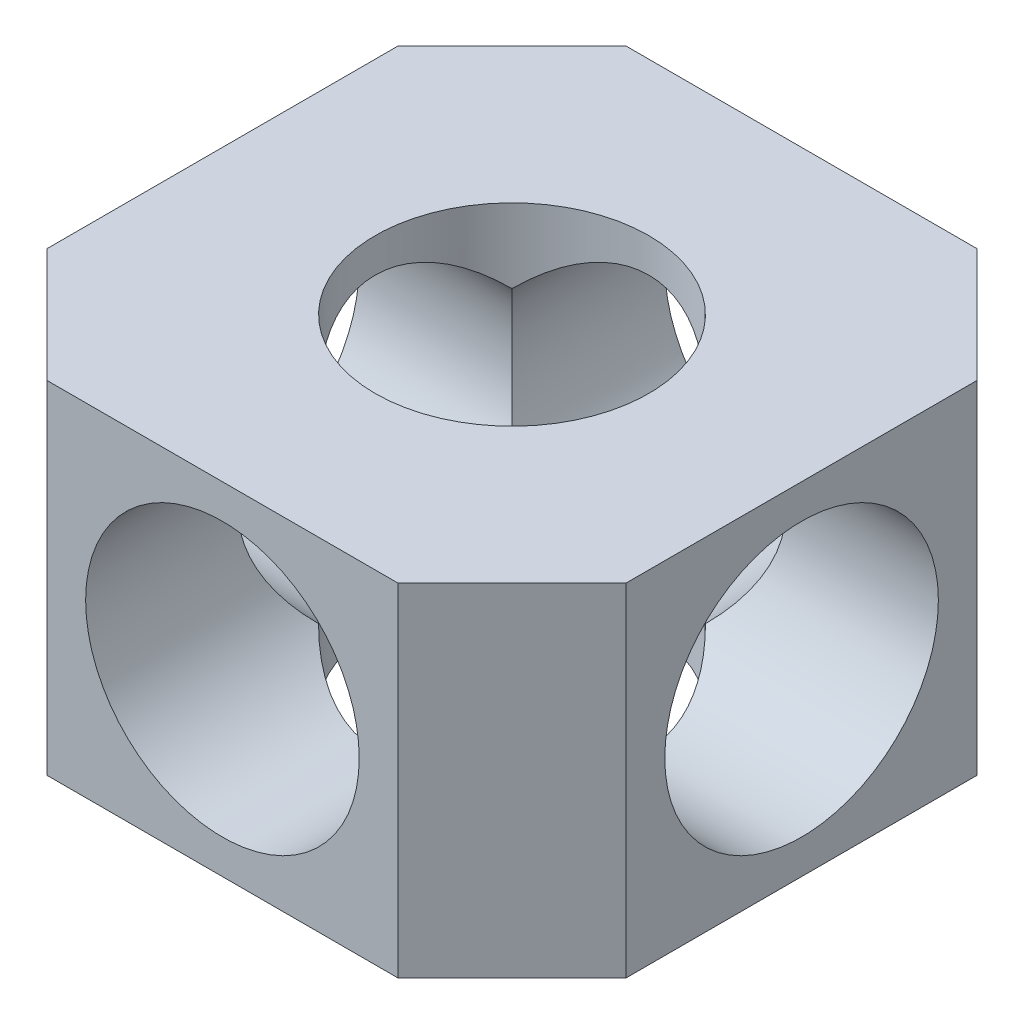
ISO-10303-21;
HEADER;
FILE_DESCRIPTION(('STEP AP214'),'2;1');
FILE_NAME('part.step','',(''),(''),'','','');
FILE_SCHEMA(('AUTOMOTIVE_DESIGN { 1 0 10303 214 1 1 1 1 }'));
ENDSEC;
DATA;
#1=APPLICATION_CONTEXT('core data for automotive mechanical design processes');
#2=APPLICATION_PROTOCOL_DEFINITION('international standard','automotive_design',2000,#1);
#3=PRODUCT_CONTEXT('',#1,'mechanical');
#4=PRODUCT('Part','Part','',(#3));
#5=PRODUCT_RELATED_PRODUCT_CATEGORY('part','',(#4));
#6=PRODUCT_DEFINITION_FORMATION('','',#4);
#7=PRODUCT_DEFINITION_CONTEXT('part definition',#1,'design');
#8=PRODUCT_DEFINITION('design','',#6,#7);
#9=PRODUCT_DEFINITION_SHAPE('','',#8);
#10=(LENGTH_UNIT() NAMED_UNIT(*) SI_UNIT(.MILLI.,.METRE.));
#11=(NAMED_UNIT(*) PLANE_ANGLE_UNIT() SI_UNIT($,.RADIAN.));
#12=(NAMED_UNIT(*) SI_UNIT($,.STERADIAN.) SOLID_ANGLE_UNIT());
#13=UNCERTAINTY_MEASURE_WITH_UNIT(LENGTH_MEASURE(1.E-05),#10,'distance_accuracy_value','');
#14=(GEOMETRIC_REPRESENTATION_CONTEXT(3) GLOBAL_UNCERTAINTY_ASSIGNED_CONTEXT((#13)) GLOBAL_UNIT_ASSIGNED_CONTEXT((#10,
#11,#12)) REPRESENTATION_CONTEXT('',''));
#15=CARTESIAN_POINT('',(0.,0.,0.));
#16=DIRECTION('',(0.,0.,1.));
#17=DIRECTION('',(1.,0.,0.));
#18=AXIS2_PLACEMENT_3D('',#15,#16,#17);
#19=CARTESIAN_POINT('',(0.,7.5,23.3));
#20=DIRECTION('',(0.,0.,-1.));
#21=DIRECTION('',(-1.,0.,0.));
#22=AXIS2_PLACEMENT_3D('',#19,#20,#21);
#23=CYLINDRICAL_SURFACE('',#22,6.);
#24=CARTESIAN_POINT('',(0.,7.5,-12.7));
#25=DIRECTION('',(0.,0.,-1.));
#26=DIRECTION('',(-1.,0.,0.));
#27=AXIS2_PLACEMENT_3D('',#24,#25,#26);
#28=CIRCLE('',#27,6.);
#29=CARTESIAN_POINT('',(-6.,7.5,-12.7));
#30=VERTEX_POINT('',#29);
#31=EDGE_CURVE('E179',#30,#30,#28,.T.);
#32=ORIENTED_EDGE('',*,*,#31,.T.);
#33=EDGE_LOOP('',(#32));
#34=FACE_BOUND('',#33,.T.);
#35=CARTESIAN_POINT('',(0.,7.5,0.));
#36=DIRECTION('',(0.707106781186547,0.,-0.707106781186548));
#37=DIRECTION('',(-0.707106781186548,0.,-0.707106781186547));
#38=AXIS2_PLACEMENT_3D('',#35,#36,#37);
#39=ELLIPSE('',#38,8.48528137423857,6.);
#40=CARTESIAN_POINT('',(-4.24264068711928,11.7426406871193,-4.24264068711928));
#41=VERTEX_POINT('',#40);
#42=CARTESIAN_POINT('',(-4.24264068711928,3.25735931288072,-4.24264068711928));
#43=VERTEX_POINT('',#42);
#44=EDGE_CURVE('E136',#41,#43,#39,.F.);
#45=ORIENTED_EDGE('',*,*,#44,.T.);
#46=CARTESIAN_POINT('',(0.,7.5,0.));
#47=DIRECTION('',(0.,0.707106781186547,-0.707106781186547));
#48=DIRECTION('',(0.,-0.707106781186547,-0.707106781186547));
#49=AXIS2_PLACEMENT_3D('',#46,#47,#48);
#50=ELLIPSE('',#49,8.48528137423857,6.);
#51=CARTESIAN_POINT('',(4.2426406871193,3.25735931288072,-4.24264068711928));
#52=VERTEX_POINT('',#51);
#53=EDGE_CURVE('E56',#43,#52,#50,.F.);
#54=ORIENTED_EDGE('',*,*,#53,.T.);
#55=CARTESIAN_POINT('',(0.,7.5,0.));
#56=DIRECTION('',(-0.707106781186548,0.,-0.707106781186547));
#57=DIRECTION('',(0.707106781186547,0.,-0.707106781186548));
#58=AXIS2_PLACEMENT_3D('',#55,#56,#57);
#59=ELLIPSE('',#58,8.48528137423857,6.);
#60=CARTESIAN_POINT('',(4.2426406871193,11.7426406871193,-4.24264068711928));
#61=VERTEX_POINT('',#60);
#62=EDGE_CURVE('E154',#52,#61,#59,.F.);
#63=ORIENTED_EDGE('',*,*,#62,.T.);
#64=CARTESIAN_POINT('',(0.,7.5,0.));
#65=DIRECTION('',(0.,-0.707106781186547,-0.707106781186547));
#66=DIRECTION('',(0.,0.707106781186547,-0.707106781186547));
#67=AXIS2_PLACEMENT_3D('',#64,#65,#66);
#68=ELLIPSE('',#67,8.48528137423857,6.);
#69=EDGE_CURVE('E162',#61,#41,#68,.F.);
#70=ORIENTED_EDGE('',*,*,#69,.T.);
#71=EDGE_LOOP('',(#45,#54,#63,#70));
#72=FACE_BOUND('',#71,.T.);
#73=ADVANCED_FACE('F43',(#34,#72),#23,.F.);
#74=CARTESIAN_POINT('',(12.7,15.,0.));
#75=DIRECTION('',(-1.,0.,0.));
#76=DIRECTION('',(0.,0.,1.));
#77=AXIS2_PLACEMENT_3D('',#74,#75,#76);
#78=PLANE('',#77);
#79=CARTESIAN_POINT('',(12.7,7.5,0.));
#80=DIRECTION('',(1.,0.,0.));
#81=DIRECTION('',(0.,0.,-1.));
#82=AXIS2_PLACEMENT_3D('',#79,#80,#81);
#83=CIRCLE('',#82,6.);
#84=CARTESIAN_POINT('',(12.7,7.5,-5.99999999999999));
#85=VERTEX_POINT('',#84);
#86=EDGE_CURVE('E172',#85,#85,#83,.T.);
#87=ORIENTED_EDGE('',*,*,#86,.F.);
#88=EDGE_LOOP('',(#87));
#89=FACE_BOUND('',#88,.T.);
#90=DIRECTION('',(0.,0.,-1.));
#91=VECTOR('',#90,1.);
#92=CARTESIAN_POINT('',(12.7,0.,0.));
#93=LINE('',#92,#91);
#94=CARTESIAN_POINT('',(12.7,0.,7.7));
#95=VERTEX_POINT('',#94);
#96=CARTESIAN_POINT('',(12.7,0.,-7.69999999999998));
#97=VERTEX_POINT('',#96);
#98=EDGE_CURVE('E196',#95,#97,#93,.T.);
#99=ORIENTED_EDGE('',*,*,#98,.T.);
#100=DIRECTION('',(0.,1.,0.));
#101=VECTOR('',#100,1.);
#102=CARTESIAN_POINT('',(12.7,15.,-7.69999999999998));
#103=LINE('',#102,#101);
#104=CARTESIAN_POINT('',(12.7,15.,-7.69999999999998));
#105=VERTEX_POINT('',#104);
#106=EDGE_CURVE('E225',#97,#105,#103,.T.);
#107=ORIENTED_EDGE('',*,*,#106,.T.);
#108=DIRECTION('',(0.,0.,-1.));
#109=VECTOR('',#108,1.);
#110=CARTESIAN_POINT('',(12.7,15.,12.7));
#111=LINE('',#110,#109);
#112=CARTESIAN_POINT('',(12.7,15.,7.7));
#113=VERTEX_POINT('',#112);
#114=EDGE_CURVE('E183',#113,#105,#111,.T.);
#115=ORIENTED_EDGE('',*,*,#114,.F.);
#116=DIRECTION('',(0.,-1.,0.));
#117=VECTOR('',#116,1.);
#118=CARTESIAN_POINT('',(12.7,15.,7.7));
#119=LINE('',#118,#117);
#120=EDGE_CURVE('E199',#113,#95,#119,.T.);
#121=ORIENTED_EDGE('',*,*,#120,.T.);
#122=EDGE_LOOP('',(#99,#107,#115,#121));
#123=FACE_BOUND('',#122,.T.);
#124=ADVANCED_FACE('F264',(#89,#123),#78,.F.);
#125=CARTESIAN_POINT('',(12.7,15.,-12.7));
#126=DIRECTION('',(0.,0.,1.));
#127=DIRECTION('',(1.,0.,0.));
#128=AXIS2_PLACEMENT_3D('',#125,#126,#127);
#129=PLANE('',#128);
#130=ORIENTED_EDGE('',*,*,#31,.F.);
#131=EDGE_LOOP('',(#130));
#132=FACE_BOUND('',#131,.T.);
#133=DIRECTION('',(-1.,0.,0.));
#134=VECTOR('',#133,1.);
#135=CARTESIAN_POINT('',(12.7,0.,-12.7));
#136=LINE('',#135,#134);
#137=CARTESIAN_POINT('',(7.7,0.,-12.7));
#138=VERTEX_POINT('',#137);
#139=CARTESIAN_POINT('',(-7.69999999999998,0.,-12.7));
#140=VERTEX_POINT('',#139);
#141=EDGE_CURVE('E197',#138,#140,#136,.T.);
#142=ORIENTED_EDGE('',*,*,#141,.T.);
#143=DIRECTION('',(0.,1.,0.));
#144=VECTOR('',#143,1.);
#145=CARTESIAN_POINT('',(-7.69999999999998,15.,-12.7));
#146=LINE('',#145,#144);
#147=CARTESIAN_POINT('',(-7.69999999999998,15.,-12.7));
#148=VERTEX_POINT('',#147);
#149=EDGE_CURVE('E233',#140,#148,#146,.T.);
#150=ORIENTED_EDGE('',*,*,#149,.T.);
#151=DIRECTION('',(-1.,0.,0.));
#152=VECTOR('',#151,1.);
#153=CARTESIAN_POINT('',(12.7,15.,-12.7));
#154=LINE('',#153,#152);
#155=CARTESIAN_POINT('',(7.7,15.,-12.7));
#156=VERTEX_POINT('',#155);
#157=EDGE_CURVE('E190',#156,#148,#154,.T.);
#158=ORIENTED_EDGE('',*,*,#157,.F.);
#159=DIRECTION('',(0.,-1.,0.));
#160=VECTOR('',#159,1.);
#161=CARTESIAN_POINT('',(7.7,15.,-12.7));
#162=LINE('',#161,#160);
#163=EDGE_CURVE('E216',#156,#138,#162,.T.);
#164=ORIENTED_EDGE('',*,*,#163,.T.);
#165=EDGE_LOOP('',(#142,#150,#158,#164));
#166=FACE_BOUND('',#165,.T.);
#167=ADVANCED_FACE('F266',(#132,#166),#129,.F.);
#168=CARTESIAN_POINT('',(-12.7,15.,-12.7));
#169=DIRECTION('',(1.,0.,0.));
#170=DIRECTION('',(0.,0.,-1.));
#171=AXIS2_PLACEMENT_3D('',#168,#169,#170);
#172=PLANE('',#171);
#173=CARTESIAN_POINT('',(-12.7,7.5,0.));
#174=DIRECTION('',(1.,0.,0.));
#175=DIRECTION('',(0.,0.,-1.));
#176=AXIS2_PLACEMENT_3D('',#173,#174,#175);
#177=CIRCLE('',#176,6.);
#178=CARTESIAN_POINT('',(-12.7,7.5,-5.99999999999999));
#179=VERTEX_POINT('',#178);
#180=EDGE_CURVE('E180',#179,#179,#177,.T.);
#181=ORIENTED_EDGE('',*,*,#180,.T.);
#182=EDGE_LOOP('',(#181));
#183=FACE_BOUND('',#182,.T.);
#184=DIRECTION('',(0.,0.,1.));
#185=VECTOR('',#184,1.);
#186=CARTESIAN_POINT('',(-12.7,0.,-12.7));
#187=LINE('',#186,#185);
#188=CARTESIAN_POINT('',(-12.7,0.,-7.69999999999999));
#189=VERTEX_POINT('',#188);
#190=CARTESIAN_POINT('',(-12.7,0.,7.69999999999999));
#191=VERTEX_POINT('',#190);
#192=EDGE_CURVE('E201',#189,#191,#187,.T.);
#193=ORIENTED_EDGE('',*,*,#192,.T.);
#194=DIRECTION('',(0.,1.,0.));
#195=VECTOR('',#194,1.);
#196=CARTESIAN_POINT('',(-12.7,15.,7.69999999999999));
#197=LINE('',#196,#195);
#198=CARTESIAN_POINT('',(-12.7,15.,7.69999999999999));
#199=VERTEX_POINT('',#198);
#200=EDGE_CURVE('E239',#191,#199,#197,.T.);
#201=ORIENTED_EDGE('',*,*,#200,.T.);
#202=DIRECTION('',(0.,0.,1.));
#203=VECTOR('',#202,1.);
#204=CARTESIAN_POINT('',(-12.7,15.,-12.7));
#205=LINE('',#204,#203);
#206=CARTESIAN_POINT('',(-12.7,15.,-7.69999999999999));
#207=VERTEX_POINT('',#206);
#208=EDGE_CURVE('E192',#207,#199,#205,.T.);
#209=ORIENTED_EDGE('',*,*,#208,.F.);
#210=DIRECTION('',(0.,-1.,0.));
#211=VECTOR('',#210,1.);
#212=CARTESIAN_POINT('',(-12.7,15.,-7.69999999999999));
#213=LINE('',#212,#211);
#214=EDGE_CURVE('E228',#207,#189,#213,.T.);
#215=ORIENTED_EDGE('',*,*,#214,.T.);
#216=EDGE_LOOP('',(#193,#201,#209,#215));
#217=FACE_BOUND('',#216,.T.);
#218=ADVANCED_FACE('F273',(#183,#217),#172,.F.);
#219=CARTESIAN_POINT('',(-12.7,15.,12.7));
#220=DIRECTION('',(0.,0.,-1.));
#221=DIRECTION('',(-1.,0.,0.));
#222=AXIS2_PLACEMENT_3D('',#219,#220,#221);
#223=PLANE('',#222);
#224=CARTESIAN_POINT('',(0.,7.5,12.7));
#225=DIRECTION('',(0.,0.,-1.));
#226=DIRECTION('',(-1.,0.,0.));
#227=AXIS2_PLACEMENT_3D('',#224,#225,#226);
#228=CIRCLE('',#227,6.);
#229=CARTESIAN_POINT('',(-5.99999999999999,7.5,12.7));
#230=VERTEX_POINT('',#229);
#231=EDGE_CURVE('E182',#230,#230,#228,.T.);
#232=ORIENTED_EDGE('',*,*,#231,.T.);
#233=EDGE_LOOP('',(#232));
#234=FACE_BOUND('',#233,.T.);
#235=DIRECTION('',(1.,0.,0.));
#236=VECTOR('',#235,1.);
#237=CARTESIAN_POINT('',(-12.7,15.,12.7));
#238=LINE('',#237,#236);
#239=CARTESIAN_POINT('',(-7.69999999999999,15.,12.7));
#240=VERTEX_POINT('',#239);
#241=CARTESIAN_POINT('',(7.69999999999998,15.,12.7));
#242=VERTEX_POINT('',#241);
#243=EDGE_CURVE('E191',#240,#242,#238,.T.);
#244=ORIENTED_EDGE('',*,*,#243,.F.);
#245=DIRECTION('',(0.,-1.,0.));
#246=VECTOR('',#245,1.);
#247=CARTESIAN_POINT('',(-7.69999999999999,15.,12.7));
#248=LINE('',#247,#246);
#249=CARTESIAN_POINT('',(-7.69999999999999,0.,12.7));
#250=VERTEX_POINT('',#249);
#251=EDGE_CURVE('E232',#240,#250,#248,.T.);
#252=ORIENTED_EDGE('',*,*,#251,.T.);
#253=DIRECTION('',(1.,0.,0.));
#254=VECTOR('',#253,1.);
#255=CARTESIAN_POINT('',(-12.7,0.,12.7));
#256=LINE('',#255,#254);
#257=CARTESIAN_POINT('',(7.69999999999998,0.,12.7));
#258=VERTEX_POINT('',#257);
#259=EDGE_CURVE('E189',#250,#258,#256,.T.);
#260=ORIENTED_EDGE('',*,*,#259,.T.);
#261=DIRECTION('',(0.,1.,0.));
#262=VECTOR('',#261,1.);
#263=CARTESIAN_POINT('',(7.69999999999998,15.,12.7));
#264=LINE('',#263,#262);
#265=EDGE_CURVE('E215',#258,#242,#264,.T.);
#266=ORIENTED_EDGE('',*,*,#265,.T.);
#267=EDGE_LOOP('',(#244,#252,#260,#266));
#268=FACE_BOUND('',#267,.T.);
#269=ADVANCED_FACE('F244',(#234,#268),#223,.F.);
#270=CARTESIAN_POINT('',(0.,15.,0.));
#271=DIRECTION('',(0.,1.,0.));
#272=DIRECTION('',(0.,0.,1.));
#273=AXIS2_PLACEMENT_3D('',#270,#271,#272);
#274=PLANE('',#273);
#275=CARTESIAN_POINT('',(0.,15.,0.));
#276=DIRECTION('',(0.,1.,0.));
#277=DIRECTION('',(0.,0.,1.));
#278=AXIS2_PLACEMENT_3D('',#275,#276,#277);
#279=CIRCLE('',#278,6.);
#280=CARTESIAN_POINT('',(0.,15.,6.));
#281=VERTEX_POINT('',#280);
#282=EDGE_CURVE('E150',#281,#281,#279,.T.);
#283=ORIENTED_EDGE('',*,*,#282,.F.);
#284=EDGE_LOOP('',(#283));
#285=FACE_BOUND('',#284,.T.);
#286=ORIENTED_EDGE('',*,*,#208,.T.);
#287=DIRECTION('',(-0.707106781186546,0.,-0.707106781186549));
#288=VECTOR('',#287,1.);
#289=CARTESIAN_POINT('',(-10.2,15.,10.2));
#290=LINE('',#289,#288);
#291=EDGE_CURVE('E152',#199,#240,#290,.F.);
#292=ORIENTED_EDGE('',*,*,#291,.T.);
#293=ORIENTED_EDGE('',*,*,#243,.T.);
#294=DIRECTION('',(-0.707106781186549,0.,0.707106781186547));
#295=VECTOR('',#294,1.);
#296=CARTESIAN_POINT('',(10.2,15.,10.2));
#297=LINE('',#296,#295);
#298=EDGE_CURVE('E213',#242,#113,#297,.F.);
#299=ORIENTED_EDGE('',*,*,#298,.T.);
#300=ORIENTED_EDGE('',*,*,#114,.T.);
#301=DIRECTION('',(0.707106781186546,0.,0.707106781186549));
#302=VECTOR('',#301,1.);
#303=CARTESIAN_POINT('',(10.2,15.,-10.2));
#304=LINE('',#303,#302);
#305=EDGE_CURVE('E224',#105,#156,#304,.F.);
#306=ORIENTED_EDGE('',*,*,#305,.T.);
#307=ORIENTED_EDGE('',*,*,#157,.T.);
#308=DIRECTION('',(0.707106781186549,0.,-0.707106781186546));
#309=VECTOR('',#308,1.);
#310=CARTESIAN_POINT('',(-10.2,15.,-10.2));
#311=LINE('',#310,#309);
#312=EDGE_CURVE('E231',#148,#207,#311,.F.);
#313=ORIENTED_EDGE('',*,*,#312,.T.);
#314=EDGE_LOOP('',(#286,#292,#293,#299,#300,#306,#307,#313));
#315=FACE_BOUND('',#314,.T.);
#316=ADVANCED_FACE('F290',(#285,#315),#274,.T.);
#317=CARTESIAN_POINT('',(0.,0.,0.));
#318=DIRECTION('',(0.,1.,0.));
#319=DIRECTION('',(0.,0.,1.));
#320=AXIS2_PLACEMENT_3D('',#317,#318,#319);
#321=PLANE('',#320);
#322=CARTESIAN_POINT('',(0.,0.,0.));
#323=DIRECTION('',(0.,1.,0.));
#324=DIRECTION('',(0.,0.,1.));
#325=AXIS2_PLACEMENT_3D('',#322,#323,#324);
#326=CIRCLE('',#325,6.);
#327=CARTESIAN_POINT('',(0.,0.,6.));
#328=VERTEX_POINT('',#327);
#329=EDGE_CURVE('E168',#328,#328,#326,.T.);
#330=ORIENTED_EDGE('',*,*,#329,.T.);
#331=EDGE_LOOP('',(#330));
#332=FACE_BOUND('',#331,.T.);
#333=ORIENTED_EDGE('',*,*,#259,.F.);
#334=DIRECTION('',(0.707106781186546,0.,0.707106781186549));
#335=VECTOR('',#334,1.);
#336=CARTESIAN_POINT('',(-7.69999999999999,0.,12.7));
#337=LINE('',#336,#335);
#338=EDGE_CURVE('E238',#250,#191,#337,.F.);
#339=ORIENTED_EDGE('',*,*,#338,.T.);
#340=ORIENTED_EDGE('',*,*,#192,.F.);
#341=DIRECTION('',(-0.707106781186549,0.,0.707106781186546));
#342=VECTOR('',#341,1.);
#343=CARTESIAN_POINT('',(-12.7,0.,-7.69999999999999));
#344=LINE('',#343,#342);
#345=EDGE_CURVE('E230',#189,#140,#344,.F.);
#346=ORIENTED_EDGE('',*,*,#345,.T.);
#347=ORIENTED_EDGE('',*,*,#141,.F.);
#348=DIRECTION('',(-0.707106781186546,0.,-0.707106781186549));
#349=VECTOR('',#348,1.);
#350=CARTESIAN_POINT('',(7.69999999999999,0.,-12.7));
#351=LINE('',#350,#349);
#352=EDGE_CURVE('E217',#138,#97,#351,.F.);
#353=ORIENTED_EDGE('',*,*,#352,.T.);
#354=ORIENTED_EDGE('',*,*,#98,.F.);
#355=DIRECTION('',(0.707106781186549,0.,-0.707106781186547));
#356=VECTOR('',#355,1.);
#357=CARTESIAN_POINT('',(12.7,0.,7.7));
#358=LINE('',#357,#356);
#359=EDGE_CURVE('E209',#95,#258,#358,.F.);
#360=ORIENTED_EDGE('',*,*,#359,.T.);
#361=EDGE_LOOP('',(#333,#339,#340,#346,#347,#353,#354,#360));
#362=FACE_BOUND('',#361,.T.);
#363=ADVANCED_FACE('F310',(#332,#362),#321,.F.);
#364=CARTESIAN_POINT('',(12.7,15.,7.7));
#365=DIRECTION('',(-0.707106781186547,0.,-0.707106781186549));
#366=DIRECTION('',(0.,-1.,0.));
#367=AXIS2_PLACEMENT_3D('',#364,#365,#366);
#368=PLANE('',#367);
#369=ORIENTED_EDGE('',*,*,#298,.F.);
#370=ORIENTED_EDGE('',*,*,#265,.F.);
#371=ORIENTED_EDGE('',*,*,#359,.F.);
#372=ORIENTED_EDGE('',*,*,#120,.F.);
#373=EDGE_LOOP('',(#369,#370,#371,#372));
#374=FACE_BOUND('',#373,.T.);
#375=ADVANCED_FACE('F299',(#374),#368,.F.);
#376=CARTESIAN_POINT('',(7.69999999999999,15.,-12.7));
#377=DIRECTION('',(-0.707106781186549,0.,0.707106781186546));
#378=DIRECTION('',(0.,-1.,0.));
#379=AXIS2_PLACEMENT_3D('',#376,#377,#378);
#380=PLANE('',#379);
#381=ORIENTED_EDGE('',*,*,#305,.F.);
#382=ORIENTED_EDGE('',*,*,#106,.F.);
#383=ORIENTED_EDGE('',*,*,#352,.F.);
#384=ORIENTED_EDGE('',*,*,#163,.F.);
#385=EDGE_LOOP('',(#381,#382,#383,#384));
#386=FACE_BOUND('',#385,.T.);
#387=ADVANCED_FACE('F306',(#386),#380,.F.);
#388=CARTESIAN_POINT('',(-12.7,15.,-7.69999999999999));
#389=DIRECTION('',(0.707106781186546,0.,0.707106781186549));
#390=DIRECTION('',(0.,-1.,0.));
#391=AXIS2_PLACEMENT_3D('',#388,#389,#390);
#392=PLANE('',#391);
#393=ORIENTED_EDGE('',*,*,#312,.F.);
#394=ORIENTED_EDGE('',*,*,#149,.F.);
#395=ORIENTED_EDGE('',*,*,#345,.F.);
#396=ORIENTED_EDGE('',*,*,#214,.F.);
#397=EDGE_LOOP('',(#393,#394,#395,#396));
#398=FACE_BOUND('',#397,.T.);
#399=ADVANCED_FACE('F260',(#398),#392,.F.);
#400=CARTESIAN_POINT('',(-7.69999999999999,15.,12.7));
#401=DIRECTION('',(0.707106781186549,0.,-0.707106781186546));
#402=DIRECTION('',(0.,-1.,0.));
#403=AXIS2_PLACEMENT_3D('',#400,#401,#402);
#404=PLANE('',#403);
#405=ORIENTED_EDGE('',*,*,#291,.F.);
#406=ORIENTED_EDGE('',*,*,#200,.F.);
#407=ORIENTED_EDGE('',*,*,#338,.F.);
#408=ORIENTED_EDGE('',*,*,#251,.F.);
#409=EDGE_LOOP('',(#405,#406,#407,#408));
#410=FACE_BOUND('',#409,.T.);
#411=ADVANCED_FACE('F46',(#410),#404,.F.);
#412=CARTESIAN_POINT('',(0.,7.5,0.));
#413=DIRECTION('',(-0.707106781186548,0.,-0.707106781186547));
#414=DIRECTION('',(0.707106781186547,0.,-0.707106781186548));
#415=AXIS2_PLACEMENT_3D('',#412,#413,#414);
#416=ELLIPSE('',#415,8.48528137423857,6.);
#417=CARTESIAN_POINT('',(-4.24264068711928,3.25735931288072,4.2426406871193));
#418=VERTEX_POINT('',#417);
#419=CARTESIAN_POINT('',(-4.24264068711928,11.7426406871193,4.2426406871193));
#420=VERTEX_POINT('',#419);
#421=EDGE_CURVE('E144',#418,#420,#416,.T.);
#422=ORIENTED_EDGE('',*,*,#421,.T.);
#423=CARTESIAN_POINT('',(0.,7.5,0.));
#424=DIRECTION('',(0.,0.707106781186547,-0.707106781186547));
#425=DIRECTION('',(0.,-0.707106781186547,-0.707106781186547));
#426=AXIS2_PLACEMENT_3D('',#423,#424,#425);
#427=ELLIPSE('',#426,8.48528137423857,6.);
#428=CARTESIAN_POINT('',(4.24264068711929,11.7426406871193,4.24264068711929));
#429=VERTEX_POINT('',#428);
#430=EDGE_CURVE('E66',#420,#429,#427,.T.);
#431=ORIENTED_EDGE('',*,*,#430,.T.);
#432=CARTESIAN_POINT('',(0.,7.5,0.));
#433=DIRECTION('',(0.707106781186547,0.,-0.707106781186548));
#434=DIRECTION('',(-0.707106781186548,0.,-0.707106781186547));
#435=AXIS2_PLACEMENT_3D('',#432,#433,#434);
#436=ELLIPSE('',#435,8.48528137423857,6.);
#437=CARTESIAN_POINT('',(4.24264068711929,3.25735931288071,4.24264068711929));
#438=VERTEX_POINT('',#437);
#439=EDGE_CURVE('E147',#429,#438,#436,.T.);
#440=ORIENTED_EDGE('',*,*,#439,.T.);
#441=CARTESIAN_POINT('',(0.,7.5,0.));
#442=DIRECTION('',(0.,-0.707106781186547,-0.707106781186547));
#443=DIRECTION('',(0.,0.707106781186547,-0.707106781186547));
#444=AXIS2_PLACEMENT_3D('',#441,#442,#443);
#445=ELLIPSE('',#444,8.48528137423857,6.);
#446=EDGE_CURVE('E131',#438,#418,#445,.T.);
#447=ORIENTED_EDGE('',*,*,#446,.T.);
#448=EDGE_LOOP('',(#422,#431,#440,#447));
#449=FACE_BOUND('',#448,.T.);
#450=ORIENTED_EDGE('',*,*,#231,.F.);
#451=EDGE_LOOP('',(#450));
#452=FACE_BOUND('',#451,.T.);
#453=ADVANCED_FACE('F145',(#449,#452),#23,.F.);
#454=CARTESIAN_POINT('',(-23.3,7.5,0.));
#455=DIRECTION('',(1.,0.,0.));
#456=DIRECTION('',(0.,0.,-1.));
#457=AXIS2_PLACEMENT_3D('',#454,#455,#456);
#458=CYLINDRICAL_SURFACE('',#457,6.);
#459=ORIENTED_EDGE('',*,*,#86,.T.);
#460=EDGE_LOOP('',(#459));
#461=FACE_BOUND('',#460,.T.);
#462=ORIENTED_EDGE('',*,*,#62,.F.);
#463=CARTESIAN_POINT('',(0.,7.5,0.));
#464=DIRECTION('',(0.707106781186547,0.707106781186547,0.));
#465=DIRECTION('',(0.707106781186547,-0.707106781186547,0.));
#466=AXIS2_PLACEMENT_3D('',#463,#464,#465);
#467=ELLIPSE('',#466,8.48528137423857,6.);
#468=EDGE_CURVE('E166',#52,#438,#467,.F.);
#469=ORIENTED_EDGE('',*,*,#468,.T.);
#470=ORIENTED_EDGE('',*,*,#439,.F.);
#471=CARTESIAN_POINT('',(0.,7.5,0.));
#472=DIRECTION('',(0.707106781186547,-0.707106781186547,0.));
#473=DIRECTION('',(0.707106781186547,0.707106781186547,0.));
#474=AXIS2_PLACEMENT_3D('',#471,#472,#473);
#475=ELLIPSE('',#474,8.48528137423857,6.);
#476=EDGE_CURVE('E165',#429,#61,#475,.F.);
#477=ORIENTED_EDGE('',*,*,#476,.T.);
#478=EDGE_LOOP('',(#462,#469,#470,#477));
#479=FACE_BOUND('',#478,.T.);
#480=ADVANCED_FACE('F247',(#461,#479),#458,.F.);
#481=ORIENTED_EDGE('',*,*,#44,.F.);
#482=CARTESIAN_POINT('',(0.,7.5,0.));
#483=DIRECTION('',(0.707106781186547,0.707106781186547,0.));
#484=DIRECTION('',(0.707106781186547,-0.707106781186547,0.));
#485=AXIS2_PLACEMENT_3D('',#482,#483,#484);
#486=ELLIPSE('',#485,8.48528137423857,6.);
#487=EDGE_CURVE('E11',#41,#420,#486,.T.);
#488=ORIENTED_EDGE('',*,*,#487,.T.);
#489=ORIENTED_EDGE('',*,*,#421,.F.);
#490=CARTESIAN_POINT('',(0.,7.5,0.));
#491=DIRECTION('',(0.707106781186547,-0.707106781186547,0.));
#492=DIRECTION('',(0.707106781186547,0.707106781186547,0.));
#493=AXIS2_PLACEMENT_3D('',#490,#491,#492);
#494=ELLIPSE('',#493,8.48528137423857,6.);
#495=EDGE_CURVE('E55',#418,#43,#494,.T.);
#496=ORIENTED_EDGE('',*,*,#495,.T.);
#497=EDGE_LOOP('',(#481,#488,#489,#496));
#498=FACE_BOUND('',#497,.T.);
#499=ORIENTED_EDGE('',*,*,#180,.F.);
#500=EDGE_LOOP('',(#499));
#501=FACE_BOUND('',#500,.T.);
#502=ADVANCED_FACE('F146',(#498,#501),#458,.F.);
#503=CARTESIAN_POINT('',(0.,-21.,0.));
#504=DIRECTION('',(0.,1.,0.));
#505=DIRECTION('',(0.,0.,1.));
#506=AXIS2_PLACEMENT_3D('',#503,#504,#505);
#507=CYLINDRICAL_SURFACE('',#506,6.);
#508=ORIENTED_EDGE('',*,*,#53,.F.);
#509=ORIENTED_EDGE('',*,*,#495,.F.);
#510=ORIENTED_EDGE('',*,*,#446,.F.);
#511=ORIENTED_EDGE('',*,*,#468,.F.);
#512=EDGE_LOOP('',(#508,#509,#510,#511));
#513=FACE_BOUND('',#512,.T.);
#514=ORIENTED_EDGE('',*,*,#329,.F.);
#515=EDGE_LOOP('',(#514));
#516=FACE_BOUND('',#515,.T.);
#517=ADVANCED_FACE('F128',(#513,#516),#507,.F.);
#518=ORIENTED_EDGE('',*,*,#282,.T.);
#519=EDGE_LOOP('',(#518));
#520=FACE_BOUND('',#519,.T.);
#521=ORIENTED_EDGE('',*,*,#430,.F.);
#522=ORIENTED_EDGE('',*,*,#487,.F.);
#523=ORIENTED_EDGE('',*,*,#69,.F.);
#524=ORIENTED_EDGE('',*,*,#476,.F.);
#525=EDGE_LOOP('',(#521,#522,#523,#524));
#526=FACE_BOUND('',#525,.T.);
#527=ADVANCED_FACE('F414',(#520,#526),#507,.F.);
#528=CLOSED_SHELL('',(#73,#124,#167,#218,#269,#316,#363,#375,#387,#399,#411,#453,#480,#502,#517,#527));
#529=MANIFOLD_SOLID_BREP('B2',#528);
#530=ADVANCED_BREP_SHAPE_REPRESENTATION('',(#18,#529),#14);
#531=SHAPE_DEFINITION_REPRESENTATION(#9,#530);
ENDSEC;
END-ISO-10303-21;
